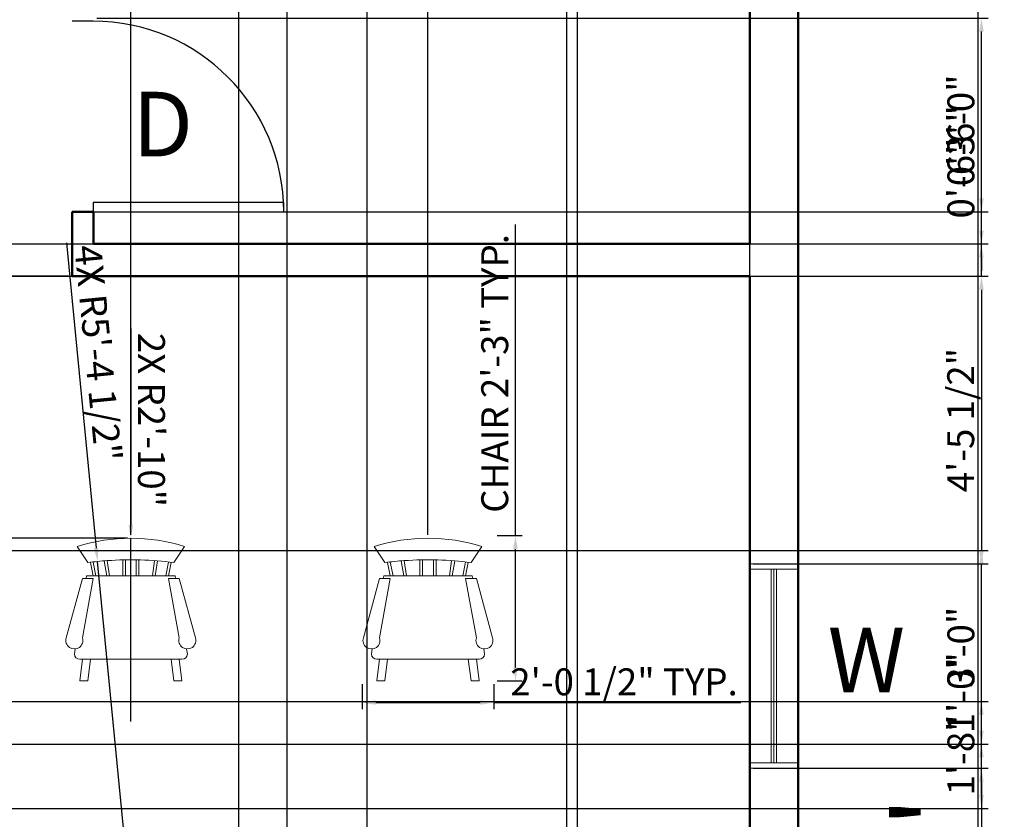
# Model space of a CAD drawing. Units: inches. Extents: x 2050 to 2529, y 1266 to 1968.
# Tile 4 of 5: x 2310 to 2493, y 1585 to 1733. Entities that reach past the tile are written whole.
import ezdxf

# ---------------------------------------------------------------- set-up
doc = ezdxf.new("R2010")
doc.units = ezdxf.units.IN
for name, color, linetype, lineweight in [('A-ANNO-DIMS', 2, 'Continuous', 18), ('A-ANNO-TEXT', 7, 'Continuous', 18), ('A-DOOR', 3, 'Continuous', 25), ('A-FURN', 8, 'Continuous', 18), ('A-GLAZ', 4, 'Continuous', 18), ('A-WALL', 7, 'Continuous', 50)]:
    doc.layers.add(name, color=color, linetype=linetype, lineweight=lineweight)
doc.styles.get("Standard").update_dxf_attribs({"font": 'arial.ttf'})
doc.dimstyles.new('ISO-25', dxfattribs={"dimtxt": 5, "dimasz": 2.5, "dimexe": 1.25, "dimexo": 0.625, "dimtad": 1, "dimlunit": 3, "dimtxsty": 'Standard', "dimcen": 2.5, "dimadec": 0, "dimazin": 0, "dimtfac": 1, "dimtmove": 0, "dimatfit": 3, "dimfxl": 1, "dimarcsym": 0})

# ---------------------------------------------------------------- blocks, each defined once
blk = doc.blocks.new('*D2')
at = {"layer": 'A-ANNO-DIMS', "color": 0, "lineweight": -2, "transparency": 16777216}
for p, q in [((2454.92, 1844.72), (2488.97, 1844.72)), ((2487.72, 1842.22), (2487.72, 1307.22)), ((2454.92, 1304.72), (2488.97, 1304.72))]:
    blk.add_line(p, q, dxfattribs=at)
at = {"layer": 'A-ANNO-DIMS', "color": 0, "transparency": 16777216}
for points in [[(2487.3, 1842.22), (2488.13, 1842.22), (2487.72, 1844.72)], [(2487.3, 1307.22), (2488.13, 1307.22), (2487.72, 1304.72)]]:
    blk.add_solid(points, dxfattribs=at)
at = {"layer": 'Defpoints', "color": 0, "transparency": 16777216}
for p in [(2454.29, 1844.72), (2454.29, 1304.72), (2487.72, 1304.72)]:
    blk.add_point(p, dxfattribs=at)
at = {"layer": 'A-ANNO-DIMS', "color": 0, "transparency": 16777216, "insert": (2479.46, 1574.72), "char_height": 5, "attachment_point": 5, "rotation": 90}
blk.add_mtext("{\\H3x;45'}", dxfattribs=at)
blk = doc.blocks.new('*U7')
for p, q in [((0, 0), (0, -100)), ((-900, 0), (-900, -100))]:
    blk.add_line(p, q)
blk.add_lwpolyline([(0, 0), (0, 900), (-43.75, 900), (-43.75, 0)], close=True)
blk.add_arc((0, 0), 900, 90, 180)
blk = doc.blocks.new('Chair - Rocking')
for p, q in [((-8, -4.5), (-10, -1.5)), ((8, -4.5), (10, -1.5)), ((-7.5, -4.5), (-7, -7)), ((-6.5, -7), (-7.02225, -4.43)), ((-4.5, -7), (-4.96674, -4.19951)), ((-4, -7), (-4.40532, -4.16272)), ((-1.5, -4.05012), (-1.5, -7)), ((-1, -7), (-1, -4.05012)), ((1, -7), (1, -4.04655)), ((1.5, -4.05012), (1.5, -7)), ((4, -7), (4.40187, -4.18694)), ((4.5, -7), (4.96761, -4.19437)), ((6.5, -7), (7, -4.4057)), ((7.5, -4.5), (7, -7)), ((-8.23428, -6.99939), (-8.3093, -7.47958)), ((-8.23041, -7), (8.23915, -7)), ((8.31071, -7.48854), (8.23449, -7.00073)), ((-9, -7.5), (-12, -18.49999)), ((-7, -7.5), (-9, -7.5)), ((-9, -18.49999), (-7, -7.5)), ((7, -7.5), (9, -7.5)), ((9, -18.49999), (7, -7.5)), ((9, -7.5), (12, -18.49999)), ((-10.36644, -20.64523), (-10.5, -21.49999)), ((10.5, -21.49999), (10.3575, -20.58798)), ((-9, -22.49999), (-9.5, -26.49999)), ((0, -22.49999), (-9.5, -22.49999)), ((-8, -26.49999), (-7.5, -22.49999)), ((0, -22.49999), (9.5, -22.49999)), ((8, -26.49999), (7.5, -22.49999)), ((9, -22.49999), (9.5, -26.49999)), ((-9.5, -26.49999), (-8, -26.49999)), ((9.5, -26.49999), (8, -26.49999))]:
    blk.add_line(p, q)
for centre, radius, start, end in [((0, -34.08333), 34.08333, 72.93847, 107.0615), ((0, -68.25004), 64.25, 93.92211, 97.15267), ((0, -68.25004), 64.25, 82.84733, 93.92211), ((-10.5, -18.99999), 1.58114, 161.5651, 18.43495), ((10.5, -18.99999), 1.58114, 161.5651, 18.43495), ((-9.5, -21.49999), 1, 180, 270), ((9.5, -21.49999), 1, 270, 0)]:
    blk.add_arc(centre, radius, start, end)
blk = doc.blocks.new('WIN-36IN')
for p, q in [((0, 9), (0, 0)), ((1, 9), (1, 0)), ((37, 9), (37, 0)), ((38, 9), (38, 0)), ((1, 5), (37, 5)), ((1, 4.5), (37, 4.5)), ((1, 4), (37, 4))]:
    blk.add_line(p, q)
blk = doc.blocks.new('*D30')
at = {"layer": 'A-ANNO-DIMS', "color": 0, "lineweight": -2, "transparency": 16777216}
for p, q in [((2401.74, 1637.48), (2401.74, 1695.32)), ((2398.31, 1637.48), (2402.99, 1637.48)), ((2401.74, 1612.98), (2401.74, 1634.98)), ((2398.31, 1610.48), (2402.99, 1610.48))]:
    blk.add_line(p, q, dxfattribs=at)
at = {"layer": 'A-ANNO-DIMS', "color": 0, "transparency": 16777216}
for points in [[(2401.32, 1634.98), (2402.16, 1634.98), (2401.74, 1637.48)], [(2401.32, 1612.98), (2402.16, 1612.98), (2401.74, 1610.48)]]:
    blk.add_solid(points, dxfattribs=at)
at = {"layer": 'Defpoints', "color": 0, "transparency": 16777216}
for p in [(2397.69, 1637.48), (2401.74, 1637.48), (2397.69, 1610.48)]:
    blk.add_point(p, dxfattribs=at)
at = {"layer": 'A-ANNO-DIMS', "color": 0, "transparency": 16777216, "insert": (2398.53, 1667.65), "char_height": 5, "attachment_point": 5, "rotation": 90}
blk.add_mtext('CHAIR 2\'-3" TYP.', dxfattribs=at)
blk = doc.blocks.new('*D31')
at = {"layer": 'A-ANNO-DIMS', "color": 0, "lineweight": -2, "transparency": 16777216}
for p, q in [((2373.25, 1609.86), (2373.25, 1605.18)), ((2397.69, 1609.86), (2397.69, 1605.18)), ((2375.75, 1606.43), (2395.19, 1606.43)), ((2397.69, 1606.43), (2443.65, 1606.43))]:
    blk.add_line(p, q, dxfattribs=at)
at = {"layer": 'A-ANNO-DIMS', "color": 0, "transparency": 16777216}
for points in [[(2375.75, 1606.85), (2375.75, 1606.02), (2373.25, 1606.43)], [(2395.19, 1606.85), (2395.19, 1606.02), (2397.69, 1606.43)]]:
    blk.add_solid(points, dxfattribs=at)
at = {"layer": 'Defpoints', "color": 0, "transparency": 16777216}
for p in [(2373.25, 1610.48), (2397.69, 1610.48), (2397.69, 1606.43)]:
    blk.add_point(p, dxfattribs=at)
at = {"layer": 'A-ANNO-DIMS', "color": 0, "transparency": 16777216, "insert": (2421.92, 1609.64), "char_height": 5, "attachment_point": 5}
blk.add_mtext('2\'-0 1/2" TYP.', dxfattribs=at)
blk = doc.blocks.new('*D44')
at = {"layer": 'A-ANNO-DIMS', "color": 0, "lineweight": -2, "transparency": 16777216}
for p, q in [((2104.36, 1606.66), (2489.62, 1606.66)), ((2488.37, 1589.22), (2488.37, 1604.16)), ((2103.92, 1586.72), (2489.62, 1586.72))]:
    blk.add_line(p, q, dxfattribs=at)
at = {"layer": 'A-ANNO-DIMS', "color": 0, "transparency": 16777216}
for points in [[(2487.95, 1604.16), (2488.79, 1604.16), (2488.37, 1606.66)], [(2487.95, 1589.22), (2488.79, 1589.22), (2488.37, 1586.72)]]:
    blk.add_solid(points, dxfattribs=at)
at = {"layer": 'Defpoints', "color": 0, "transparency": 16777216}
for p in [(2103.73, 1606.66), (2488.37, 1606.66), (2103.29, 1586.72)]:
    blk.add_point(p, dxfattribs=at)
at = {"layer": 'A-ANNO-DIMS', "color": 0, "transparency": 16777216, "insert": (2485.19, 1596.69), "char_height": 5, "attachment_point": 5, "rotation": 90}
blk.add_mtext('1\'-8"', dxfattribs=at)
blk = doc.blocks.new('*D45')
at = {"layer": 'A-ANNO-DIMS', "color": 0, "lineweight": -2, "transparency": 16777216}
for p, q in [((2259.92, 1634.72), (2489.62, 1634.72)), ((2488.37, 1601.22), (2488.37, 1632.22)), ((2259.92, 1598.72), (2489.62, 1598.72))]:
    blk.add_line(p, q, dxfattribs=at)
at = {"layer": 'A-ANNO-DIMS', "color": 0, "transparency": 16777216}
for points in [[(2487.95, 1632.22), (2488.79, 1632.22), (2488.37, 1634.72)], [(2487.95, 1601.22), (2488.79, 1601.22), (2488.37, 1598.72)]]:
    blk.add_solid(points, dxfattribs=at)
at = {"layer": 'Defpoints', "color": 0, "transparency": 16777216}
for p in [(2259.29, 1634.72), (2488.37, 1634.72), (2259.29, 1598.72)]:
    blk.add_point(p, dxfattribs=at)
at = {"layer": 'A-ANNO-DIMS', "color": 0, "transparency": 16777216, "insert": (2485.19, 1616.72), "char_height": 5, "attachment_point": 5, "rotation": 90}
blk.add_mtext('3\'-0"', dxfattribs=at)
blk = doc.blocks.new('*D47')
at = {"layer": 'A-ANNO-DIMS', "color": 0, "lineweight": -2, "transparency": 16777216}
for p, q in [((2488.37, 1598.72), (2488.37, 1615.29)), ((2259.92, 1598.72), (2489.62, 1598.72)), ((2488.37, 1589.22), (2488.37, 1596.22)), ((2259.92, 1586.72), (2489.62, 1586.72))]:
    blk.add_line(p, q, dxfattribs=at)
at = {"layer": 'A-ANNO-DIMS', "color": 0, "transparency": 16777216}
for points in [[(2487.95, 1596.22), (2488.79, 1596.22), (2488.37, 1598.72)], [(2487.95, 1589.22), (2488.79, 1589.22), (2488.37, 1586.72)]]:
    blk.add_solid(points, dxfattribs=at)
at = {"layer": 'Defpoints', "color": 0, "transparency": 16777216}
for p in [(2259.29, 1598.72), (2488.37, 1598.72), (2259.29, 1586.72)]:
    blk.add_point(p, dxfattribs=at)
at = {"layer": 'A-ANNO-DIMS', "color": 0, "transparency": 16777216, "insert": (2485.19, 1608.26), "char_height": 5, "attachment_point": 5, "rotation": 90}
blk.add_mtext('1\'-0"', dxfattribs=at)
blk = doc.blocks.new('*D48')
at = {"layer": 'A-ANNO-DIMS', "color": 0, "lineweight": -2, "transparency": 16777216}
for p, q in [((2488.37, 1694.22), (2488.37, 1711.26)), ((2259.92, 1691.72), (2489.62, 1691.72)), ((2488.37, 1685.72), (2488.37, 1691.72)), ((2259.92, 1685.72), (2489.62, 1685.72)), ((2488.37, 1683.22), (2488.37, 1680.72))]:
    blk.add_line(p, q, dxfattribs=at)
at = {"layer": 'A-ANNO-DIMS', "color": 0, "transparency": 16777216}
for points in [[(2487.95, 1694.22), (2488.79, 1694.22), (2488.37, 1691.72)], [(2487.95, 1683.22), (2488.79, 1683.22), (2488.37, 1685.72)]]:
    blk.add_solid(points, dxfattribs=at)
at = {"layer": 'Defpoints', "color": 0, "transparency": 16777216}
for p in [(2259.29, 1691.72), (2488.37, 1691.72), (2259.29, 1685.72)]:
    blk.add_point(p, dxfattribs=at)
at = {"layer": 'A-ANNO-DIMS', "color": 0, "transparency": 16777216, "insert": (2485.19, 1703.99), "char_height": 5, "attachment_point": 5, "rotation": 90}
blk.add_mtext('0\'-6"', dxfattribs=at)
blk = doc.blocks.new('*D51')
at = {"layer": 'A-ANNO-DIMS', "color": 0, "lineweight": -2, "transparency": 16777216}
for p, q in [((2413.29, 1314.35), (2413.29, 1907.05)), ((2442.79, 1905.8), (2415.79, 1905.8)), ((2445.29, 1314.35), (2445.29, 1907.05))]:
    blk.add_line(p, q, dxfattribs=at)
at = {"layer": 'A-ANNO-DIMS', "color": 0, "transparency": 16777216}
for points in [[(2415.79, 1906.21), (2415.79, 1905.38), (2413.29, 1905.8)], [(2442.79, 1906.21), (2442.79, 1905.38), (2445.29, 1905.8)]]:
    blk.add_solid(points, dxfattribs=at)
at = {"layer": 'Defpoints', "color": 0, "transparency": 16777216}
for p in [(2413.29, 1905.8), (2413.29, 1313.72), (2445.29, 1313.72)]:
    blk.add_point(p, dxfattribs=at)
at = {"layer": 'A-ANNO-DIMS', "color": 0, "transparency": 16777216, "insert": (2429.29, 1908.97), "char_height": 5, "attachment_point": 5}
blk.add_mtext('2\'-8"', dxfattribs=at)
blk = doc.blocks.new('*D52')
at = {"layer": 'A-ANNO-DIMS', "color": 0, "lineweight": -2, "transparency": 16777216}
for p, q in [((2350.29, 1390.35), (2350.29, 1907.05)), ((2352.79, 1905.8), (2356.79, 1905.8)), ((2359.29, 1390.35), (2359.29, 1907.05)), ((2359.29, 1905.8), (2376.34, 1905.8))]:
    blk.add_line(p, q, dxfattribs=at)
at = {"layer": 'A-ANNO-DIMS', "color": 0, "transparency": 16777216}
for points in [[(2352.79, 1906.21), (2352.79, 1905.38), (2350.29, 1905.8)], [(2356.79, 1906.21), (2356.79, 1905.38), (2359.29, 1905.8)]]:
    blk.add_solid(points, dxfattribs=at)
at = {"layer": 'Defpoints', "color": 0, "transparency": 16777216}
for p in [(2359.29, 1905.8), (2350.29, 1389.72), (2359.29, 1389.72)]:
    blk.add_point(p, dxfattribs=at)
at = {"layer": 'A-ANNO-DIMS', "color": 0, "transparency": 16777216, "insert": (2369.07, 1908.97), "char_height": 5, "attachment_point": 5}
blk.add_mtext('0\'-9"', dxfattribs=at)
blk = doc.blocks.new('*D56')
at = {"layer": 'A-ANNO-DIMS', "color": 0, "lineweight": -2, "transparency": 16777216}
for p, q in [((2323.92, 1733.72), (2489.62, 1733.72)), ((2488.37, 1700.22), (2488.37, 1731.22)), ((2323.92, 1697.72), (2489.62, 1697.72))]:
    blk.add_line(p, q, dxfattribs=at)
at = {"layer": 'A-ANNO-DIMS', "color": 0, "transparency": 16777216}
for points in [[(2487.95, 1731.22), (2488.79, 1731.22), (2488.37, 1733.72)], [(2487.95, 1700.22), (2488.79, 1700.22), (2488.37, 1697.72)]]:
    blk.add_solid(points, dxfattribs=at)
at = {"layer": 'Defpoints', "color": 0, "transparency": 16777216}
for p in [(2323.29, 1733.72), (2488.37, 1733.72), (2323.29, 1697.72)]:
    blk.add_point(p, dxfattribs=at)
at = {"layer": 'A-ANNO-DIMS', "color": 0, "transparency": 16777216, "insert": (2485.19, 1715.72), "char_height": 5, "attachment_point": 5, "rotation": 90}
blk.add_mtext('3\'-0"', dxfattribs=at)
blk = doc.blocks.new('*D57')
at = {"layer": 'A-ANNO-DIMS', "color": 0, "lineweight": -2, "transparency": 16777216}
for p, q in [((2488.37, 1700.22), (2488.37, 1717.26)), ((2323.92, 1697.72), (2489.62, 1697.72)), ((2488.37, 1691.72), (2488.37, 1697.72)), ((2323.92, 1691.72), (2489.62, 1691.72)), ((2488.37, 1689.22), (2488.37, 1686.72))]:
    blk.add_line(p, q, dxfattribs=at)
at = {"layer": 'A-ANNO-DIMS', "color": 0, "transparency": 16777216}
for points in [[(2487.95, 1700.22), (2488.79, 1700.22), (2488.37, 1697.72)], [(2487.95, 1689.22), (2488.79, 1689.22), (2488.37, 1691.72)]]:
    blk.add_solid(points, dxfattribs=at)
at = {"layer": 'Defpoints', "color": 0, "transparency": 16777216}
for p in [(2323.29, 1697.72), (2488.37, 1697.72), (2323.29, 1691.72)]:
    blk.add_point(p, dxfattribs=at)
at = {"layer": 'A-ANNO-DIMS', "color": 0, "transparency": 16777216, "insert": (2485.19, 1709.99), "char_height": 5, "attachment_point": 5, "rotation": 90}
blk.add_mtext('0\'-6"', dxfattribs=at)
blk = doc.blocks.new('*D71')
at = {"layer": 'A-ANNO-DIMS', "color": 0, "lineweight": -2, "transparency": 16777216}
for p, q in [((2445.92, 1685.72), (2489.62, 1685.72)), ((2488.37, 1683.22), (2488.37, 1634.72)), ((2445.92, 1632.22), (2489.62, 1632.22))]:
    blk.add_line(p, q, dxfattribs=at)
at = {"layer": 'A-ANNO-DIMS', "color": 0, "transparency": 16777216}
for points in [[(2487.95, 1683.22), (2488.79, 1683.22), (2488.37, 1685.72)], [(2487.95, 1634.72), (2488.79, 1634.72), (2488.37, 1632.22)]]:
    blk.add_solid(points, dxfattribs=at)
at = {"layer": 'Defpoints', "color": 0, "transparency": 16777216}
for p in [(2445.29, 1685.72), (2445.29, 1632.22), (2488.37, 1632.22)]:
    blk.add_point(p, dxfattribs=at)
at = {"layer": 'A-ANNO-DIMS', "color": 0, "transparency": 16777216, "insert": (2485.16, 1658.97), "char_height": 5, "attachment_point": 5, "rotation": 90}
blk.add_mtext('4\'-5 1/2"', dxfattribs=at)
blk = doc.blocks.new('*D72')
at = {"layer": 'A-ANNO-DIMS', "color": 0, "lineweight": -2, "transparency": 16777216}
for p, q in [((2445.92, 1594.22), (2489.62, 1594.22)), ((2488.37, 1591.72), (2488.37, 1489.72)), ((2445.92, 1487.22), (2489.62, 1487.22))]:
    blk.add_line(p, q, dxfattribs=at)
at = {"layer": 'A-ANNO-DIMS', "color": 0, "transparency": 16777216}
for points in [[(2487.95, 1591.72), (2488.79, 1591.72), (2488.37, 1594.22)], [(2487.95, 1489.72), (2488.79, 1489.72), (2488.37, 1487.22)]]:
    blk.add_solid(points, dxfattribs=at)
at = {"layer": 'Defpoints', "color": 0, "transparency": 16777216}
for p in [(2445.29, 1594.22), (2445.29, 1487.22), (2488.37, 1487.22)]:
    blk.add_point(p, dxfattribs=at)
at = {"layer": 'A-ANNO-DIMS', "color": 0, "transparency": 16777216, "insert": (2485.19, 1540.72), "char_height": 5, "attachment_point": 5, "rotation": 90}
blk.add_mtext('8\'-11"', dxfattribs=at)
blk = doc.blocks.new('*D77')
at = {"layer": 'A-ANNO-DIMS', "color": 0, "lineweight": -2, "transparency": 16777216}
for p, q in [((2330.24, 1637.61), (2330.24, 1907.05)), ((2332.74, 1905.8), (2382.97, 1905.8)), ((2385.47, 1637.61), (2385.47, 1907.05))]:
    blk.add_line(p, q, dxfattribs=at)
at = {"layer": 'A-ANNO-DIMS', "color": 0, "transparency": 16777216}
for points in [[(2332.74, 1906.21), (2332.74, 1905.38), (2330.24, 1905.8)], [(2382.97, 1906.21), (2382.97, 1905.38), (2385.47, 1905.8)]]:
    blk.add_solid(points, dxfattribs=at)
at = {"layer": 'Defpoints', "color": 0, "transparency": 16777216}
for p in [(2385.47, 1905.8), (2330.24, 1636.98), (2385.47, 1636.98)]:
    blk.add_point(p, dxfattribs=at)
at = {"layer": 'A-ANNO-DIMS', "color": 0, "transparency": 16777216, "insert": (2357.86, 1908.92), "char_height": 5, "attachment_point": 5}
blk.add_mtext('4\'-7"', dxfattribs=at)
blk = doc.blocks.new('*D78')
at = {"layer": 'A-ANNO-DIMS', "color": 0, "lineweight": -2, "transparency": 16777216}
for p, q in [((2318.67, 1685.72), (2058.97, 1685.72)), ((2060.22, 1683.22), (2060.22, 1639.48)), ((2329.62, 1636.98), (2058.97, 1636.98))]:
    blk.add_line(p, q, dxfattribs=at)
at = {"layer": 'A-ANNO-DIMS', "color": 0, "transparency": 16777216}
for points in [[(2059.8, 1683.22), (2060.64, 1683.22), (2060.22, 1685.72)], [(2059.8, 1639.48), (2060.64, 1639.48), (2060.22, 1636.98)]]:
    blk.add_solid(points, dxfattribs=at)
at = {"layer": 'Defpoints', "color": 0, "transparency": 16777216}
for p in [(2319.29, 1685.72), (2060.22, 1636.98), (2330.24, 1636.98)]:
    blk.add_point(p, dxfattribs=at)
at = {"layer": 'A-ANNO-DIMS', "color": 0, "transparency": 16777216, "insert": (2057.01, 1661.35), "char_height": 5, "attachment_point": 5, "rotation": 90}
blk.add_mtext('4\'-0 1/2"', dxfattribs=at)
blk = doc.blocks.new('*D79')
at = {"layer": 'A-ANNO-DIMS', "color": 0, "lineweight": -2, "transparency": 16777216}
for p, q in [((2374.17, 1568.26), (2374.17, 1907.05)), ((2376.67, 1905.8), (2408.79, 1905.8)), ((2411.29, 1583.35), (2411.29, 1907.05))]:
    blk.add_line(p, q, dxfattribs=at)
at = {"layer": 'A-ANNO-DIMS', "color": 0, "transparency": 16777216}
for points in [[(2376.67, 1906.21), (2376.67, 1905.38), (2374.17, 1905.8)], [(2408.79, 1906.21), (2408.79, 1905.38), (2411.29, 1905.8)]]:
    blk.add_solid(points, dxfattribs=at)
at = {"layer": 'Defpoints', "color": 0, "transparency": 16777216}
for p in [(2411.29, 1905.8), (2411.29, 1582.72), (2374.17, 1567.64)]:
    blk.add_point(p, dxfattribs=at)
at = {"layer": 'A-ANNO-DIMS', "color": 0, "transparency": 16777216, "insert": (2392.73, 1908.98), "char_height": 5, "attachment_point": 5}
blk.add_mtext('3\'-1"', dxfattribs=at)
blk = doc.blocks.new('*D82')
at = {"layer": 'A-ANNO-DIMS', "color": 0, "lineweight": -2, "transparency": 16777216}
for p, q in [((2318.3, 1691.92), (2323.8, 1635.17)), ((2330.24, 1568.73), (2324.04, 1632.68))]:
    blk.add_line(p, q, dxfattribs=at)
at = {"layer": 'A-ANNO-DIMS', "color": 0, "transparency": 16777216}
blk.add_solid([(2324.21, 1635.21), (2323.38, 1635.13), (2324.04, 1632.68)], dxfattribs=at)
at = {"layer": 'Defpoints', "color": 0, "transparency": 16777216}
for p in [(2324.04, 1632.68), (2330.24, 1568.73)]:
    blk.add_point(p, dxfattribs=at)
at = {"layer": 'A-ANNO-DIMS', "color": 0, "transparency": 16777216, "insert": (2323.52, 1671.36), "char_height": 5, "attachment_point": 5, "rotation": 275.5377}
blk.add_mtext('4X R5\'-4 1/2"', dxfattribs=at)
blk = doc.blocks.new('*D85')
at = {"layer": 'A-ANNO-DIMS', "color": 0, "lineweight": -2, "transparency": 16777216}
for p, q in [((2330.24, 1676.02), (2330.24, 1639.48)), ((2330.24, 1602.9), (2330.24, 1636.98))]:
    blk.add_line(p, q, dxfattribs=at)
at = {"layer": 'A-ANNO-DIMS', "color": 0, "transparency": 16777216}
blk.add_solid([(2330.66, 1639.48), (2329.82, 1639.48), (2330.24, 1636.98)], dxfattribs=at)
at = {"layer": 'Defpoints', "color": 0, "transparency": 16777216}
for p in [(2330.24, 1636.98), (2330.24, 1602.9)]:
    blk.add_point(p, dxfattribs=at)
at = {"layer": 'A-ANNO-DIMS', "color": 0, "transparency": 16777216, "insert": (2333.42, 1659), "char_height": 5, "attachment_point": 5, "rotation": 270.0003}
blk.add_mtext('2X R2\'-10"', dxfattribs=at)

msp = doc.modelspace()

# ---------------------------------------------------------------- linework, layer by layer
at = {"layer": 'A-WALL'}
for p, q in [((2454.295, 1844.72), (2454.295, 1304.72)), ((2445.295, 1835.72), (2445.295, 1691.72)), ((2319.295, 1685.72), (2319.295, 1697.72)), ((2319.295, 1697.72), (2323.295, 1697.72)), ((2323.295, 1691.72), (2323.295, 1697.72)), ((2323.295, 1691.72), (2445.295, 1691.72)), ((2319.295, 1685.72), (2445.295, 1685.72)), ((2445.295, 1685.72), (2445.295, 1395.72))]:
    msp.add_line(p, q, dxfattribs=at)

# ---------------------------------------------------------------- block references
at = {"layer": 'A-DOOR', "xscale": 0.0393700787401575, "yscale": 0.0393700787401575, "zscale": 0.0393700787401575, "rotation": 270}
msp.add_blockref('*U7', (2323.232, 1697.72), dxfattribs=at)
at = {"layer": 'A-FURN'}
for p in [(2330.24, 1636.982), (2385.471, 1636.982)]:
    msp.add_blockref('Chair - Rocking', p, dxfattribs=at)
at = {"layer": 'A-GLAZ', "rotation": 269.9999999999999}
msp.add_blockref('WIN-36IN', (2445.294, 1632.22), dxfattribs=at)

# ---------------------------------------------------------------- texts
at = {"layer": 'A-ANNO-TEXT', "char_height": 12, "attachment_point": 1}
for s, insert in [('D', (2330.528, 1720.023)), ('W', (2459.787, 1620.351))]:
    msp.add_mtext_dynamic_manual_height_columns(s, width=471.52273, gutter_width=12.5, heights=[28.462], dxfattribs=dict(at, insert=insert))

# ---------------------------------------------------------------- dimensions: what is measured, and where the dimension line sits
at = {"layer": 'A-ANNO-DIMS'}
for base, p1, p2, picture, middle in [((2385.471, 1905.795), (2330.24, 1636.982), (2385.471, 1636.982), '*D77', (2357.856, 1908.92)), ((2359.295, 1905.795), (2350.295, 1389.72), (2359.295, 1389.72), '*D52', (2369.065, 1908.973)), ((2411.295, 1905.795), (2374.175, 1567.637), (2411.295, 1582.72), '*D79', (2392.735, 1908.975)), ((2413.295, 1905.795), (2445.295, 1313.72), (2413.295, 1313.72), '*D51', (2429.295, 1908.973))]:
    dim = msp.add_linear_dim(base=base, p1=p1, p2=p2, dimstyle='ISO-25', override={"dimdec": 1, "dimlfac": 1, "dimrnd": 0, "dimzin": 1, "dimdsep": 46, "dimlunit": 4, "dimfrac": 2}, dxfattribs=at)
    dim.commit()
    dim.dimension.update_dxf_attribs({"geometry": picture, "text_midpoint": middle})
for base, p1, p2, text, override, picture, middle in [((2487.716, 1304.72), (2454.295, 1844.72), (2454.295, 1304.72), '{\\H3x;<>}', {"dimclrd": 0, "dimclre": 0, "dimclrt": 0}, '*D2', (2479.463, 1574.72)), ((2401.739, 1637.482), (2397.689, 1610.482), (2397.689, 1637.482), 'CHAIR <> TYP.', {"dimdec": 1, "dimlfac": 1, "dimrnd": 0, "dimzin": 1, "dimdsep": 46, "dimlunit": 4, "dimfrac": 2}, '*D30', (2398.527, 1667.654))]:
    dim = msp.add_linear_dim(base=base, p1=p1, p2=p2, angle=90, text=text, dimstyle='ISO-25', override=override, dxfattribs=at)
    dim.commit()
    dim.dimension.update_dxf_attribs({"geometry": picture, "text_midpoint": middle})
for base, p1, p2, picture, middle in [((2488.37, 1733.72), (2323.295, 1697.72), (2323.295, 1733.72), '*D56', (2485.19, 1715.72)), ((2488.37, 1697.72), (2323.295, 1691.72), (2323.295, 1697.72), '*D57', (2485.192, 1709.991)), ((2488.37, 1691.72), (2259.295, 1685.72), (2259.295, 1691.72), '*D48', (2485.192, 1703.991)), ((2060.22, 1636.982), (2319.295, 1685.72), (2330.24, 1636.982), '*D78', (2057.009, 1661.351)), ((2488.37, 1632.22), (2445.295, 1685.72), (2445.295, 1632.22), '*D71', (2485.159, 1658.97)), ((2488.37, 1634.72), (2259.295, 1598.72), (2259.295, 1634.72), '*D45', (2485.19, 1616.72)), ((2488.37, 1598.72), (2259.295, 1586.72), (2259.295, 1598.72), '*D47', (2485.192, 1608.256)), ((2488.37, 1606.66), (2103.295, 1586.72), (2103.734, 1606.66), '*D44', (2485.192, 1596.69)), ((2488.37, 1487.22), (2445.295, 1594.22), (2445.295, 1487.22), '*D72', (2485.192, 1540.72))]:
    dim = msp.add_linear_dim(base=base, p1=p1, p2=p2, angle=90, dimstyle='ISO-25', override={"dimdec": 1, "dimlfac": 1, "dimrnd": 0, "dimzin": 1, "dimdsep": 46, "dimlunit": 4, "dimfrac": 2}, dxfattribs=at)
    dim.commit()
    dim.dimension.update_dxf_attribs({"geometry": picture, "text_midpoint": middle})
dim = msp.add_radius_dim(center=(2330.24017, 1568.73218), mpoint=(2324.03997, 1632.68232), text='4X <>', dimstyle='ISO-25', override={"dimdec": 1, "dimlfac": 1, "dimrnd": 0, "dimzin": 1, "dimdsep": 46, "dimlunit": 4, "dimfrac": 2}, dxfattribs=at)
dim.commit()
dim.dimension.update_dxf_attribs({"geometry": '*D82', "text_midpoint": (2320.31985, 1671.0524), "dimtype": 164})
dim = msp.add_radius_dim(center=(2330.24, 1602.899), mpoint=(2330.24, 1636.982), text='2X <>', dimstyle='ISO-25', override={"dimdec": 1, "dimlfac": 1, "dimrnd": 0, "dimzin": 1, "dimdsep": 46, "dimlunit": 4, "dimfrac": 2}, dxfattribs=at)
dim.commit()
dim.dimension.update_dxf_attribs({"geometry": '*D85', "text_midpoint": (2333.418, 1659.002)})
dim = msp.add_linear_dim(base=(2397.689, 1606.432), p1=(2373.253, 1610.482), p2=(2397.689, 1610.482), text='<> TYP.', dimstyle='ISO-25', override={"dimdec": 1, "dimlfac": 1, "dimrnd": 0, "dimzin": 1, "dimdsep": 46, "dimlunit": 4, "dimfrac": 2}, dxfattribs=at)
dim.commit()
dim.dimension.update_dxf_attribs({"geometry": '*D31', "text_midpoint": (2421.92, 1609.643)})

doc.saveas('drawing.dxf')
